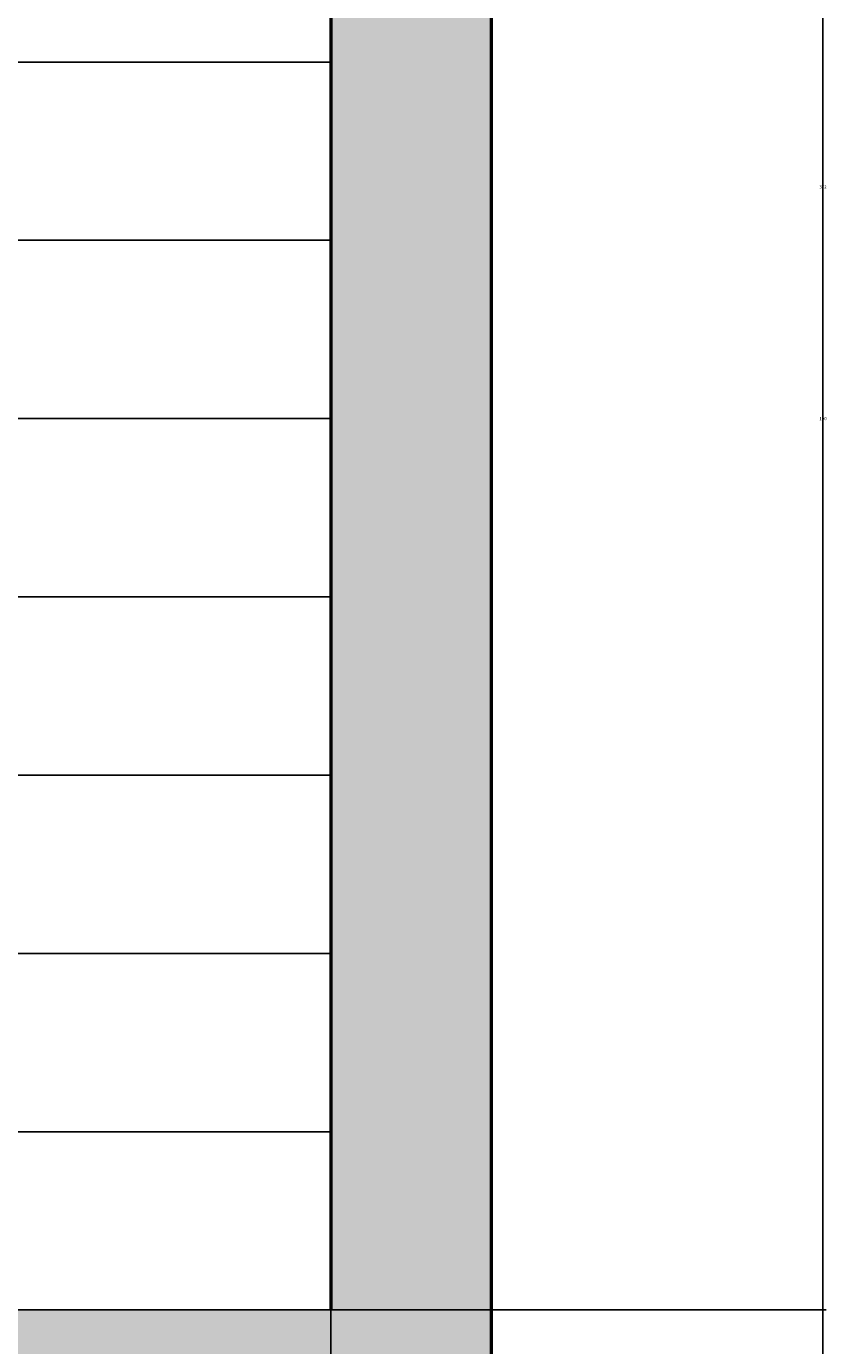
# Model space of a CAD drawing. Units: inches. Extents: x 2231 to 2461, y 2045 to 2455.
# Tile 60 of 95: x 2416 to 2461, y 2185 to 2259. Entities that reach past the tile are written whole.
import ezdxf

# ---------------------------------------------------------------- set-up
doc = ezdxf.new("R2010")
doc.units = ezdxf.units.IN
for name, color, linetype, lineweight in [('A-ANNO-DIMS', 2, 'Continuous', 18), ('A-FLOR-STRS', 7, 'Continuous', 25), ('A-WALL', 7, 'Continuous', 50)]:
    doc.layers.add(name, color=color, linetype=linetype, lineweight=lineweight)
doc.layers.add('A-WALL-PATT', color=18, linetype='Continuous', lineweight=13, true_color=0x000000)
doc.styles.get("Standard").update_dxf_attribs({"font": 'arial.ttf'})
doc.dimstyles.get("Standard").update_dxf_attribs({"dimtxt": 0.18, "dimasz": 0.18, "dimexe": 0.18, "dimexo": 0.0625, "dimgap": 0.09, "dimtad": 0, "dimtih": 1, "dimtoh": 1, "dimdec": 4, "dimzin": 0, "dimdsep": 46, "dimtxsty": 'Standard', "dimcen": 0.09, "dimadec": 0, "dimazin": 0, "dimtfac": 1, "dimtdec": 4, "dimtofl": 0, "dimtmove": 0, "dimatfit": 3, "dimfxl": 1, "dimtolj": 1, "dimtzin": 0, "dimarcsym": 0})

# ---------------------------------------------------------------- blocks, each defined once
blk = doc.blocks.new('*D34')
at = {"layer": 'A-ANNO-DIMS', "color": 0, "lineweight": -2, "transparency": 16777216}
for p, q in [((2441.856, 2435.833), (2460.606, 2435.833)), ((2460.426, 2435.653), (2460.426, 2250.015)), ((2460.426, 2064.013), (2460.426, 2249.651)), ((2441.856, 2063.833), (2460.606, 2063.833))]:
    blk.add_line(p, q, dxfattribs=at)
at = {"layer": 'A-ANNO-DIMS', "color": 0, "transparency": 16777216}
for points in [[(2460.396, 2435.653), (2460.456, 2435.653), (2460.426, 2435.833)], [(2460.396, 2064.013), (2460.456, 2064.013), (2460.426, 2063.833)]]:
    blk.add_solid(points, dxfattribs=at)
at = {"layer": 'Defpoints', "color": 0, "transparency": 16777216}
for p in [(2441.794, 2435.833), (2460.426, 2435.833), (2441.794, 2063.833)]:
    blk.add_point(p, dxfattribs=at)
at = {"layer": 'A-ANNO-DIMS', "color": 0, "transparency": 16777216, "insert": (2460.426, 2249.833), "char_height": 0.18, "attachment_point": 5}
blk.add_mtext('\\A1;372', dxfattribs=at)
blk = doc.blocks.new('*D43')
at = {"layer": 'A-ANNO-DIMS', "color": 0, "lineweight": -2, "transparency": 16777216}
for p, q in [((2432.856, 2286.833), (2460.606, 2286.833)), ((2460.426, 2286.653), (2460.426, 2237.015)), ((2460.426, 2187.013), (2460.426, 2236.651)), ((2432.856, 2186.833), (2460.606, 2186.833))]:
    blk.add_line(p, q, dxfattribs=at)
at = {"layer": 'A-ANNO-DIMS', "color": 0, "transparency": 16777216}
for points in [[(2460.396, 2286.653), (2460.456, 2286.653), (2460.426, 2286.833)], [(2460.396, 2187.013), (2460.456, 2187.013), (2460.426, 2186.833)]]:
    blk.add_solid(points, dxfattribs=at)
at = {"layer": 'Defpoints', "color": 0, "transparency": 16777216}
for p in [(2432.794, 2286.833), (2460.426, 2286.833), (2432.794, 2186.833)]:
    blk.add_point(p, dxfattribs=at)
at = {"layer": 'A-ANNO-DIMS', "color": 0, "transparency": 16777216, "insert": (2460.426, 2236.833), "char_height": 0.18, "attachment_point": 5}
blk.add_mtext('\\A1;100', dxfattribs=at)
blk = doc.blocks.new('*D59')
at = {"layer": 'A-ANNO-DIMS', "color": 0, "lineweight": -2, "transparency": 16777216}
for p, q in [((2408.794, 2182.895), (2408.794, 2454.645)), ((2432.794, 2182.895), (2432.794, 2454.645)), ((2408.974, 2454.465), (2420.573, 2454.465)), ((2432.614, 2454.465), (2421.014, 2454.465))]:
    blk.add_line(p, q, dxfattribs=at)
at = {"layer": 'A-ANNO-DIMS', "color": 0, "transparency": 16777216}
for points in [[(2408.974, 2454.495), (2408.974, 2454.435), (2408.794, 2454.465)], [(2432.614, 2454.495), (2432.614, 2454.435), (2432.794, 2454.465)]]:
    blk.add_solid(points, dxfattribs=at)
at = {"layer": 'Defpoints', "color": 0, "transparency": 16777216}
for p in [(2432.794, 2454.465), (2408.794, 2182.833), (2432.794, 2182.833)]:
    blk.add_point(p, dxfattribs=at)
at = {"layer": 'A-ANNO-DIMS', "color": 0, "transparency": 16777216, "insert": (2420.794, 2454.465), "char_height": 0.18, "attachment_point": 5}
blk.add_mtext('\\A1;24', dxfattribs=at)

msp = doc.modelspace()

# ---------------------------------------------------------------- hatches: boundary and pattern name
at = {"layer": 'A-WALL-PATT'}
h = msp.add_hatch(color=256, dxfattribs=at)
h.dxf.hatch_style = 1
h.paths.add_polyline_path([(2441.7935, 2269.1535), (2432.7935, 2269.1535), (2432.7935, 2186.8328), (2396.7935, 2186.8328), (2396.7935, 2286.8328), (2394.7935, 2286.8328), (2394.7935, 2186.8328), (2334.7935, 2186.8328), (2334.7935, 2182.8328), (2432.7935, 2182.8328), (2432.7935, 2072.8328), (2416.6639, 2072.8328), (2416.6639, 2063.8328), (2441.7935, 2063.8328)])
h.paths.add_polyline_path([(2368.6639, 2072.8328), (2367.04, 2072.8328), (2330.7942, 2072.8328), (2330.7397, 2063.8328), (2368.6639, 2063.8328)])
h.paths.add_polyline_path([(2300.7392, 2068.3328), (2300.7392, 2072.8328), (2298.7935, 2072.8328), (2294.7935, 2072.8328), (2258.7935, 2072.8328), (2258.7935, 2120.8328), (2294.7935, 2120.8328), (2298.7935, 2120.8328), (2298.7935, 2128.8328), (2294.7935, 2128.8328), (2294.7935, 2124.8328), (2258.7935, 2124.8328), (2258.7935, 2182.8328), (2294.7935, 2182.8328), (2294.7935, 2174.8328), (2298.7935, 2174.8328), (2298.7935, 2182.8328), (2304.7935, 2182.8328), (2304.7935, 2186.8328), (2258.7935, 2186.8328), (2258.7935, 2221.999), (2249.7935, 2221.999), (2249.7935, 2063.8328), (2300.7392, 2063.8328)])
h.paths.add_polyline_path([(2391.9338, 2435.8328), (2333.82, 2435.8328), (2333.82, 2426.8328), (2368.7935, 2426.8328), (2368.7935, 2374.9508), (2368.7935, 2370.8328), (2372.3935, 2370.8328), (2372.7935, 2370.8328), (2372.7935, 2426.8328), (2391.9338, 2426.8328)])
h.paths.add_polyline_path([(2441.7935, 2435.8328), (2415.9338, 2435.8328), (2415.9338, 2426.8328), (2432.7935, 2426.8328), (2432.7935, 2334.8328), (2372.7935, 2334.8328), (2372.7935, 2346.8328), (2368.7935, 2346.8328), (2368.7935, 2306.8328), (2360.7935, 2306.8328), (2360.7935, 2302.8328), (2368.7935, 2302.8328), (2372.7935, 2302.8328), (2372.7935, 2330.8328), (2432.7935, 2330.8328), (2432.7935, 2317.1535), (2441.7935, 2317.1535)])
h.paths.add_polyline_path([(2285.82, 2435.8328), (2249.7935, 2435.8328), (2249.7935, 2269.999), (2258.7935, 2269.999), (2258.7935, 2302.8328), (2318.8168, 2302.8328), (2330.7935, 2302.8328), (2330.7935, 2306.8328), (2258.7935, 2306.8328), (2258.7935, 2426.8328), (2285.82, 2426.8328)])

# ---------------------------------------------------------------- linework, layer by layer
at = {"layer": 'A-FLOR-STRS'}
for p, q in [((2396.7935, 2256.8328), (2432.7935, 2256.8328)), ((2396.7935, 2246.8328), (2432.7935, 2246.8328)), ((2396.7935, 2236.8328), (2432.7935, 2236.8328)), ((2396.7935, 2226.8328), (2432.7935, 2226.8328)), ((2396.7935, 2216.8328), (2432.7935, 2216.8328)), ((2396.7935, 2206.8328), (2432.7935, 2206.8328)), ((2396.7935, 2196.8328), (2432.7935, 2196.8328)), ((2396.7935, 2186.8328), (2432.7935, 2186.8328))]:
    msp.add_line(p, q, dxfattribs=at)
at = {"layer": 'A-WALL'}
msp.add_line((2432.7935, 2330.8328), (2432.7935, 2186.8328), dxfattribs=at)
msp.add_lwpolyline([(2300.7392, 2063.8328), (2249.7935, 2063.8328), (2249.7935, 2435.8328), (2441.7935, 2435.8328), (2441.7935, 2063.8328), (2330.7397, 2063.8328)], dxfattribs=at)

# ---------------------------------------------------------------- dimensions: what is measured, and where the dimension line sits
at = {"layer": 'A-ANNO-DIMS'}
dim = msp.add_linear_dim(base=(2432.7935, 2454.4653), p1=(2408.7935, 2182.8328), p2=(2432.7935, 2182.8328), dimstyle='Standard', override={"dimdec": 0, "dimlfac": 1, "dimrnd": 0, "dimzin": 0, "dimdsep": 46, "dimlunit": 2}, dxfattribs=at)
dim.commit()
dim.dimension.update_dxf_attribs({"geometry": '*D59', "text_midpoint": (2420.7935, 2454.4653)})
for base, p1, p2, picture, middle in [((2460.426, 2435.8328), (2441.7935, 2063.8328), (2441.7935, 2435.8328), '*D34', (2460.426, 2249.8328)), ((2460.426, 2286.8328), (2432.7935, 2186.8328), (2432.7935, 2286.8328), '*D43', (2460.426, 2236.8328))]:
    dim = msp.add_linear_dim(base=base, p1=p1, p2=p2, angle=90, dimstyle='Standard', override={"dimdec": 0, "dimlfac": 1, "dimrnd": 0, "dimzin": 0, "dimdsep": 46, "dimlunit": 2}, dxfattribs=at)
    dim.commit()
    dim.dimension.update_dxf_attribs({"geometry": picture, "text_midpoint": middle})

doc.saveas('drawing.dxf')
